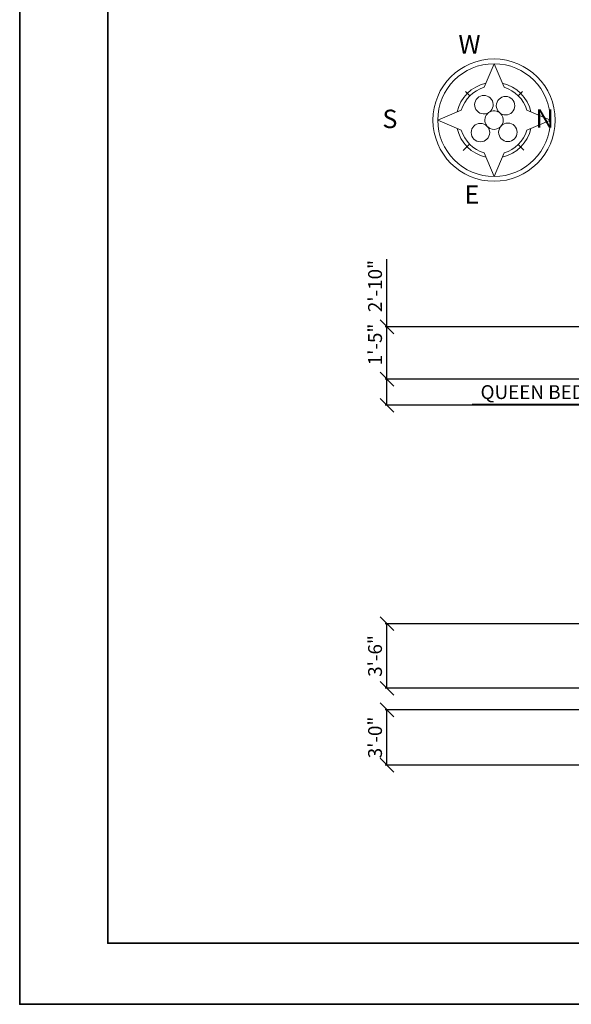
# Model space of a CAD drawing. Units: inches. Extents: x 1798 to 3594, y 1405 to 2404.
# Tile 1 of 6: x 1798 to 2157, y 1405 to 2046. Entities that reach past the tile are written whole.
import ezdxf

# ---------------------------------------------------------------- set-up
doc = ezdxf.new("R2010")
doc.units = ezdxf.units.IN
for name, color, linetype, lineweight in [('A-ANNO-DIMS', 6, 'Continuous', 18), ('A-ANNO-SYMB', 7, 'Continuous', 18), ('A-ANNO-TTLB', 7, 'Continuous', 35)]:
    doc.layers.add(name, color=color, linetype=linetype, lineweight=lineweight)
doc.styles.get("Standard").update_dxf_attribs({"font": 'arial.ttf'})
doc.dimstyles.new('ISO-25', dxfattribs={"dimtxt": 9, "dimasz": 9, "dimexe": 1.25, "dimexo": 0.625, "dimgap": 2, "dimtad": 1, "dimdec": 1, "dimlunit": 4, "dimtxsty": 'Standard', "dimblk": 'OBLIQUE', "dimcen": 2.5, "dimazin": 0, "dimtfac": 1, "dimtdec": 1, "dimtmove": 0, "dimatfit": 3, "dimfxl": 1, "dimarcsym": 0})

# ---------------------------------------------------------------- blocks, each defined once
blk = doc.blocks.new('_Oblique')
at = {"color": 0, "linetype": 'ByBlock', "lineweight": -2}
blk.add_line((-0.5, -0.5), (0.5, 0.5), dxfattribs=at)
blk = doc.blocks.new('*D19')
at = {"layer": 'A-ANNO-DIMS', "color": 0, "lineweight": -2, "transparency": 16777216}
for p, q in [((2238.18, 1795.31), (2092.79, 1795.31)), ((2238.18, 1783.93), (2238.18, 1796.56)), ((2318.18, 1795.31), (2238.18, 1795.31)), ((2318.18, 1783.93), (2318.18, 1796.56))]:
    blk.add_line(p, q, dxfattribs=at)
at = {"layer": 'Defpoints', "color": 0, "transparency": 16777216}
for p in [(2238.18, 1795.31), (2238.18, 1783.31), (2318.18, 1783.31)]:
    blk.add_point(p, dxfattribs=at)
at = {"layer": 'A-ANNO-DIMS', "color": 0, "lineweight": -2, "transparency": 16777216, "xscale": 9, "yscale": 9, "zscale": 9, "rotation": 180}
blk.add_blockref('_Oblique', (2238.18, 1795.31), dxfattribs=at)
at = {"layer": 'A-ANNO-DIMS', "color": 0, "lineweight": -2, "transparency": 16777216, "xscale": 9, "yscale": 9, "zscale": 9}
blk.add_blockref('_Oblique', (2318.18, 1795.31), dxfattribs=at)
at = {"layer": 'A-ANNO-DIMS', "color": 0, "transparency": 16777216, "insert": (2160.99, 1802.24), "char_height": 9, "attachment_point": 5}
blk.add_mtext('QUEEN BED 6\'-8" TYP.', dxfattribs=at)
blk = doc.blocks.new('*D44')
at = {"layer": 'A-ANNO-DIMS', "color": 0, "lineweight": -2, "transparency": 16777216}
for p, q in [((2037.37, 1845.81), (2037.37, 1889.88)), ((2225.65, 1845.81), (2036.12, 1845.81)), ((2037.37, 1811.81), (2037.37, 1845.81)), ((2225.65, 1811.81), (2036.12, 1811.81))]:
    blk.add_line(p, q, dxfattribs=at)
at = {"layer": 'Defpoints', "color": 0, "transparency": 16777216}
for p in [(2037.37, 1845.81), (2226.27, 1845.81), (2226.27, 1811.81)]:
    blk.add_point(p, dxfattribs=at)
at = {"layer": 'A-ANNO-DIMS', "color": 0, "lineweight": -2, "transparency": 16777216, "xscale": 9, "yscale": 9, "zscale": 9}
for p, rotation in [((2037.37, 1845.81), 90), ((2037.37, 1811.81), 270)]:
    blk.add_blockref('_Oblique', p, dxfattribs=dict(at, rotation=rotation))
at = {"layer": 'A-ANNO-DIMS', "color": 0, "transparency": 16777216, "insert": (2030.78, 1872.35), "char_height": 9, "attachment_point": 5, "rotation": 90}
blk.add_mtext('2\'-10"', dxfattribs=at)
blk = doc.blocks.new('*D45')
at = {"layer": 'A-ANNO-DIMS', "color": 0, "lineweight": -2, "transparency": 16777216}
for p, q in [((2037.37, 1811.81), (2037.37, 1847.89)), ((2225.65, 1811.81), (2036.12, 1811.81)), ((2037.37, 1794.81), (2037.37, 1811.81)), ((2234.65, 1794.81), (2036.12, 1794.81))]:
    blk.add_line(p, q, dxfattribs=at)
at = {"layer": 'Defpoints', "color": 0, "transparency": 16777216}
for p in [(2037.37, 1811.81), (2226.27, 1811.81), (2235.27, 1794.81)]:
    blk.add_point(p, dxfattribs=at)
at = {"layer": 'A-ANNO-DIMS', "color": 0, "lineweight": -2, "transparency": 16777216, "xscale": 9, "yscale": 9, "zscale": 9}
for p, rotation in [((2037.37, 1811.81), 90), ((2037.37, 1794.81), 270)]:
    blk.add_blockref('_Oblique', p, dxfattribs=dict(at, rotation=rotation))
at = {"layer": 'A-ANNO-DIMS', "color": 0, "transparency": 16777216, "insert": (2030.78, 1834.35), "char_height": 9, "attachment_point": 5, "rotation": 90}
blk.add_mtext('1\'-5"', dxfattribs=at)
blk = doc.blocks.new('*D48')
at = {"layer": 'A-ANNO-DIMS', "color": 0, "lineweight": -2, "transparency": 16777216}
for p, q in [((2225.65, 1652.81), (2036.12, 1652.81)), ((2037.37, 1610.81), (2037.37, 1652.81)), ((2225.65, 1610.81), (2036.12, 1610.81))]:
    blk.add_line(p, q, dxfattribs=at)
at = {"layer": 'Defpoints', "color": 0, "transparency": 16777216}
for p in [(2037.37, 1652.81), (2226.27, 1652.81), (2226.27, 1610.81)]:
    blk.add_point(p, dxfattribs=at)
at = {"layer": 'A-ANNO-DIMS', "color": 0, "lineweight": -2, "transparency": 16777216, "xscale": 9, "yscale": 9, "zscale": 9}
for p, rotation in [((2037.37, 1652.81), 90), ((2037.37, 1610.81), 270)]:
    blk.add_blockref('_Oblique', p, dxfattribs=dict(at, rotation=rotation))
at = {"layer": 'A-ANNO-DIMS', "color": 0, "transparency": 16777216, "insert": (2030.77, 1631.81), "char_height": 9, "attachment_point": 5, "rotation": 90}
blk.add_mtext('3\'-6"', dxfattribs=at)
blk = doc.blocks.new('*D52')
at = {"layer": 'A-ANNO-DIMS', "color": 0, "lineweight": -2, "transparency": 16777216}
for p, q in [((2270.65, 1596.81), (2036.12, 1596.81)), ((2037.37, 1560.81), (2037.37, 1596.81)), ((2234.65, 1560.81), (2036.12, 1560.81))]:
    blk.add_line(p, q, dxfattribs=at)
at = {"layer": 'Defpoints', "color": 0, "transparency": 16777216}
for p in [(2037.37, 1596.81), (2271.27, 1596.81), (2235.27, 1560.81)]:
    blk.add_point(p, dxfattribs=at)
at = {"layer": 'A-ANNO-DIMS', "color": 0, "lineweight": -2, "transparency": 16777216, "xscale": 9, "yscale": 9, "zscale": 9}
for p, rotation in [((2037.37, 1596.81), 90), ((2037.37, 1560.81), 270)]:
    blk.add_blockref('_Oblique', p, dxfattribs=dict(at, rotation=rotation))
at = {"layer": 'A-ANNO-DIMS', "color": 0, "transparency": 16777216, "insert": (2030.77, 1578.81), "char_height": 9, "attachment_point": 5, "rotation": 90}
blk.add_mtext('3\'-0"', dxfattribs=at)

msp = doc.modelspace()

# ---------------------------------------------------------------- linework, layer by layer
at = {"layer": 'A-ANNO-SYMB'}
for p, q in [((2107.04, 2016.91), (2100.54, 2001.62)), ((2107.04, 2016.91), (2113.53, 2001.62)), ((2091.26, 1996.05), (2088.49, 1998.82)), ((2122.82, 1996.05), (2125.64, 1998.87)), ((2070.36, 1980.26), (2085.68, 1986.77)), ((2143.69, 1980.26), (2128.4, 1986.75)), ((2070.36, 1980.26), (2085.68, 1973.75)), ((2102.77, 1984.51), (2102.6, 1984.68)), ((2111.26, 1984.56), (2111.29, 1984.59)), ((2143.69, 1980.26), (2128.4, 1973.76)), ((2111.28, 1975.98), (2111.25, 1976.01)), ((2087.03, 1960.46), (2091.16, 1964.57)), ((2126.4, 1960.83), (2122.79, 1964.44)), ((2107.04, 1943.61), (2100.54, 1958.9)), ((2107.04, 1943.61), (2113.53, 1958.9))]:
    msp.add_line(p, q, dxfattribs=at)
for centre, radius in [((2107.04, 1980.26), 39.76), ((2107.04, 1980.26), 36.65), ((2114.54, 1989.66), 6.02), ((2098.18, 1972.16), 6.02), ((2116.03, 1972.35), 6.02)]:
    msp.add_circle(centre, radius, dxfattribs=at)
for centre, radius, start, end in [((2107.04, 1980.26), 24.6, 102.60579, 167.36466), ((2107.04, 1980.26), 24.6, 12.60579, 77.39421), ((2107.04, 1980.26), 22.32, 106.91523, 163.05024), ((2107.04, 1980.26), 22.32, 16.91523, 73.08477), ((2100.43, 1990.3), 6.02, 307.15812, 299.47302), ((2107.04, 1980.26), 6.02, 54.79711, 217.39666), ((2107.04, 1980.26), 6.02, 227.47991, 48.0651), ((2107.04, 1980.26), 24.6, 192.63534, 257.39421), ((2107.04, 1980.26), 22.32, 196.94976, 253.08477), ((2107.04, 1980.26), 24.6, 282.60579, 347.39421), ((2107.04, 1980.26), 22.32, 286.91523, 343.08477)]:
    msp.add_arc(centre, radius, start, end, dxfattribs=at)
at = {"layer": 'A-ANNO-TTLB'}
for points in [[(1798.35, 2403.73), (3594.23, 2403.73), (3594.23, 1405.28), (1798.35, 1405.28)], [(1855.68, 2366.05), (3540.6, 2366.05), (3540.6, 1444.98), (1855.68, 1444.98)]]:
    msp.add_lwpolyline(points, close=True, dxfattribs=at)

# ---------------------------------------------------------------- texts
at = {"layer": 'A-ANNO-SYMB'}
for s, p in [('               W', (2028.85, 2023.59)), ('               S', (1979.39, 1975.07)), ('               N', (2079.08, 1975.35)), ('                E', (2029.09, 1925.84))]:
    msp.add_text(s, height=12, dxfattribs=at).set_placement(p)

# ---------------------------------------------------------------- dimensions: what is measured, and where the dimension line sits
at = {"layer": 'A-ANNO-DIMS'}
for base, p1, p2, picture, middle in [((2037.37, 1845.81), (2226.27, 1811.81), (2226.27, 1845.81), '*D44', (2030.78, 1872.35)), ((2037.37, 1811.81), (2235.27, 1794.81), (2226.27, 1811.81), '*D45', (2030.78, 1834.35)), ((2037.37, 1652.81), (2226.27, 1610.81), (2226.27, 1652.81), '*D48', (2030.77, 1631.81)), ((2037.37, 1596.81), (2235.27, 1560.81), (2271.27, 1596.81), '*D52', (2030.77, 1578.81))]:
    dim = msp.add_linear_dim(base=base, p1=p1, p2=p2, angle=90, dimstyle='ISO-25', override={"dimdec": 1, "dimlfac": 1, "dimrnd": 0, "dimzin": 1, "dimdsep": 46, "dimlunit": 4, "dimfrac": 2}, dxfattribs=at)
    dim.commit()
    dim.dimension.update_dxf_attribs({"geometry": picture, "text_midpoint": middle})
dim = msp.add_linear_dim(base=(2238.18, 1795.31), p1=(2318.18, 1783.31), p2=(2238.18, 1783.31), angle=180, text='QUEEN BED <> TYP.', dimstyle='ISO-25', override={"dimdec": 1, "dimlfac": 1, "dimrnd": 0, "dimzin": 1, "dimdsep": 46, "dimlunit": 4, "dimfrac": 2}, dxfattribs=at)
dim.commit()
dim.dimension.update_dxf_attribs({"geometry": '*D19', "text_midpoint": (2160.99, 1802.24)})

doc.saveas('drawing.dxf')
